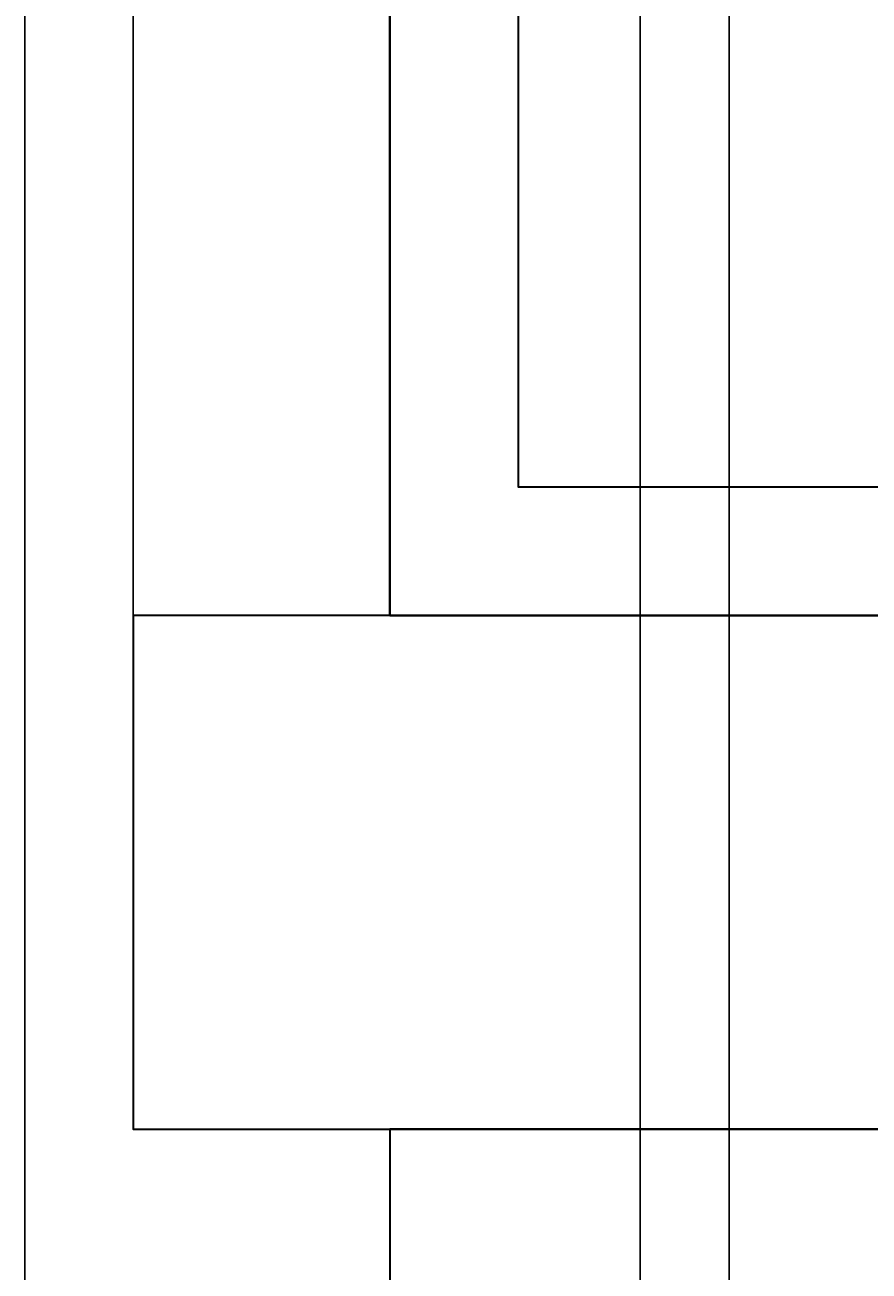
# Model space of a CAD drawing. Units: inches. Extents: x -6 to 289, y -8 to 323.
# Tile 48 of 107: x 107 to 126, y 124 to 153. Entities that reach past the tile are written whole.
import ezdxf

# ---------------------------------------------------------------- set-up
doc = ezdxf.new("R2010")
doc.units = ezdxf.units.IN
doc.header["$MEASUREMENT"] = 0
doc.layers.add('A-ANNO-DIMS', color=2, linetype='Continuous', lineweight=18)
doc.layers.add('A-ELEV', color=7, linetype='Continuous', lineweight=35)
doc.styles.get("Standard").update_dxf_attribs({"font": 'arial.ttf'})
doc.dimstyles.get("Standard").update_dxf_attribs({"dimtxt": 0.18, "dimasz": 0.18, "dimexe": 0.18, "dimexo": 0.0625, "dimgap": 0.09, "dimtad": 0, "dimtih": 1, "dimtoh": 1, "dimdec": 4, "dimzin": 0, "dimdsep": 46, "dimtxsty": 'Standard', "dimcen": 0.09, "dimadec": 0, "dimazin": 0, "dimtfac": 1, "dimtdec": 4, "dimtofl": 0, "dimtmove": 0, "dimatfit": 3, "dimfxl": 1, "dimtolj": 1, "dimtzin": 0, "dimarcsym": 0})

# ---------------------------------------------------------------- blocks, each defined once
blk = doc.blocks.new('*D58')
at = {"layer": 'A-ANNO-DIMS', "color": 0, "lineweight": -2, "transparency": 16777216}
for p, q in [((106.634, 68.495), (106.634, 322.969)), ((123.094, 68.495), (123.094, 322.969)), ((106.814, 322.789), (114.479, 322.789)), ((122.914, 322.789), (115.249, 322.789))]:
    blk.add_line(p, q, dxfattribs=at)
at = {"layer": 'A-ANNO-DIMS', "color": 0, "transparency": 16777216}
for points in [[(106.814, 322.819), (106.814, 322.759), (106.634, 322.789)], [(122.914, 322.819), (122.914, 322.759), (123.094, 322.789)]]:
    blk.add_solid(points, dxfattribs=at)
at = {"layer": 'Defpoints', "color": 0, "transparency": 16777216}
for p in [(123.094, 322.789), (106.634, 68.432), (123.094, 68.432)]:
    blk.add_point(p, dxfattribs=at)
at = {"layer": 'A-ANNO-DIMS', "color": 0, "transparency": 16777216, "insert": (114.864, 322.789), "char_height": 0.18, "attachment_point": 5}
blk.add_mtext('\\A1;16.46', dxfattribs=at)
blk = doc.blocks.new('*D73')
at = {"layer": 'A-ANNO-DIMS', "color": 0, "lineweight": -2, "transparency": 16777216}
for p, q in [((121.008, 51.148), (121.008, 322.969)), ((135.296, 51.148), (135.296, 322.969)), ((121.188, 322.789), (127.697, 322.789)), ((135.116, 322.789), (128.607, 322.789))]:
    blk.add_line(p, q, dxfattribs=at)
at = {"layer": 'A-ANNO-DIMS', "color": 0, "transparency": 16777216}
for points in [[(121.188, 322.819), (121.188, 322.759), (121.008, 322.789)], [(135.116, 322.819), (135.116, 322.759), (135.296, 322.789)]]:
    blk.add_solid(points, dxfattribs=at)
at = {"layer": 'Defpoints', "color": 0, "transparency": 16777216}
for p in [(135.296, 322.789), (121.008, 51.085), (135.296, 51.085)]:
    blk.add_point(p, dxfattribs=at)
at = {"layer": 'A-ANNO-DIMS', "color": 0, "transparency": 16777216, "insert": (128.152, 322.789), "char_height": 0.18, "attachment_point": 5}
blk.add_mtext('\\A1;14.288', dxfattribs=at)
blk = doc.blocks.new('*D92')
at = {"layer": 'A-ANNO-DIMS', "color": 0, "lineweight": -2, "transparency": 16777216}
for p, q in [((109.164, 127.351), (109.164, 322.969)), ((115.164, 162.411), (115.164, 322.969)), ((109.344, 322.789), (112.014, 322.789)), ((114.984, 322.789), (112.313, 322.789))]:
    blk.add_line(p, q, dxfattribs=at)
at = {"layer": 'A-ANNO-DIMS', "color": 0, "transparency": 16777216}
for points in [[(109.344, 322.819), (109.344, 322.759), (109.164, 322.789)], [(114.984, 322.819), (114.984, 322.759), (115.164, 322.789)]]:
    blk.add_solid(points, dxfattribs=at)
at = {"layer": 'Defpoints', "color": 0, "transparency": 16777216}
for p in [(115.164, 322.789), (115.164, 162.348), (109.164, 127.289)]:
    blk.add_point(p, dxfattribs=at)
at = {"layer": 'A-ANNO-DIMS', "color": 0, "transparency": 16777216, "insert": (112.164, 322.789), "char_height": 0.18, "attachment_point": 5}
blk.add_mtext('\\A1;6', dxfattribs=at)

msp = doc.modelspace()

# ---------------------------------------------------------------- linework, layer by layer
at = {"layer": 'A-ELEV'}
for p, q in [((115.1638, 247.2888), (115.1638, 139.2888)), ((115.1638, 139.2888), (259.1638, 139.2888)), ((259.1638, 127.2888), (115.1638, 127.2888)), ((115.1638, 127.2888), (259.1638, 127.2888)), ((115.1638, 127.2888), (115.1638, 68.4322))]:
    msp.add_line(p, q, dxfattribs=at)
for points in [[(247.1638, 139.2888), (115.1638, 139.2888), (115.1638, 162.3484), (247.1638, 162.3484)], [(244.1638, 142.2888), (118.1638, 142.2888), (118.1638, 159.3484), (244.1638, 159.3484)]]:
    msp.add_lwpolyline(points, close=True, dxfattribs=at)
msp.add_lwpolyline([(115.1638, 139.2888), (109.1638, 139.2888), (109.1638, 127.2888), (115.1638, 127.2888)], dxfattribs=at)

# ---------------------------------------------------------------- dimensions: what is measured, and where the dimension line sits
at = {"layer": 'A-ANNO-DIMS'}
for base, p1, p2, override, picture, middle in [((123.094, 322.7888), (106.634, 68.4322), (123.094, 68.4322), {"dimdec": 2, "dimlfac": 1, "dimrnd": 0, "dimzin": 0, "dimdsep": 46, "dimlunit": 2}, '*D58', (114.864, 322.7888)), ((115.1638, 322.7888), (109.1638, 127.2888), (115.1638, 162.3484), {"dimdec": 0, "dimlfac": 1, "dimrnd": 0, "dimzin": 0, "dimdsep": 46, "dimlunit": 2}, '*D92', (112.1638, 322.7888)), ((135.296, 322.7888), (121.008, 51.0851), (135.296, 51.0851), {"dimdec": 3, "dimlfac": 1, "dimrnd": 0, "dimzin": 0, "dimdsep": 46, "dimlunit": 2}, '*D73', (128.152, 322.7888))]:
    dim = msp.add_linear_dim(base=base, p1=p1, p2=p2, dimstyle='Standard', override=override, dxfattribs=at)
    dim.commit()
    dim.dimension.update_dxf_attribs({"geometry": picture, "text_midpoint": middle})

doc.saveas('drawing.dxf')
